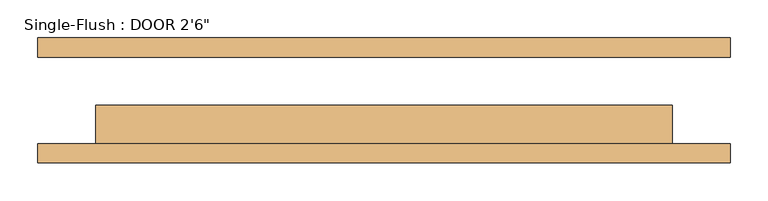
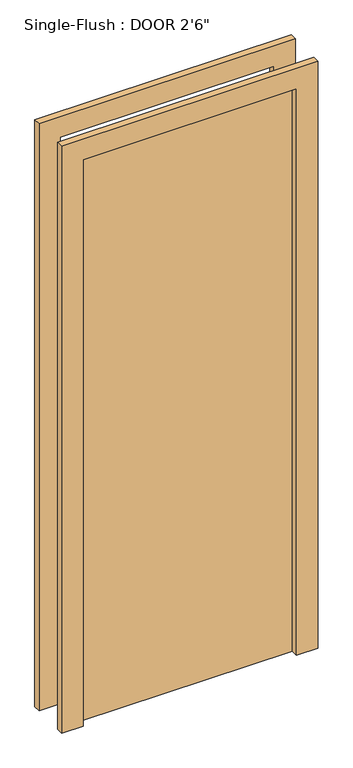
"""IFC4 building model written with IfcOpenShell, lengths in millimetres: door geometry."""

from ifc_helpers import new_model, si_unit, frame, origin, origin_with_axes, place, context, project, spatial, polyline, outline, extrude, source, transform, mapped, element, save


def door_78caadf7(model_context):
    return source(origin(), model_context, "Body", "SweptSolid", [
        extrude(outline(polyline([(2209.8, -457.2), (0.0, -457.2), (0.0, -381.0), (2133.6, -381.0), (2133.6, 381.0), (0.0, 381.0), (0.0, 457.2), (2209.8, 457.2), (2209.8, -457.2)])), frame((0.0, -82.55, 0.0), z_axis=(0.0, 1.0, 0.0), x_axis=(0.0, 0.0, 1.0)), (0.0, 0.0, 1.0), 25.4),
        extrude(outline(polyline([(2209.8, 457.2), (2209.8, -457.2), (0.0, -457.2), (0.0, -381.0), (2133.6, -381.0), (2133.6, 381.0), (0.0, 381.0), (0.0, 457.2), (2209.8, 457.2)])), frame((0.0, 57.15, 0.0), z_axis=(0.0, 1.0, 0.0), x_axis=(0.0, 0.0, 1.0)), (0.0, 0.0, 1.0), 25.4),
        extrude(outline(polyline([(381.0, -6.35), (381.0, -57.15), (-381.0, -57.15), (-381.0, -6.35), (381.0, -6.35)])), origin_with_axes(), (0.0, 0.0, 1.0), 2133.6),
    ])


if __name__ == "__main__":
    model = new_model("IFC4")
    model_context = context("Model", 3, world=origin())
    ifc_project = project(units=[si_unit("LENGTHUNIT", "METRE", prefix="MILLI")], contexts=[model_context])
    site = spatial("IfcSite", under=ifc_project)
    building = spatial("IfcBuilding", under=site)
    placement = place(None, origin())
    door_shape = door_78caadf7(model_context)
    element("IfcDoor", 1, ObjectType="Single-Flush : DOOR 2'6\"", at=placement, inside=building, context=model_context, shape_type="MappedRepresentation", body=[
        mapped(door_shape, transform((0.0, 0.0, 0.0), x_axis=(1.0, 0.0, 0.0), y_axis=(0.0, 1.0, 0.0), z_axis=(0.0, 0.0, 1.0))),
    ])
    save(model, "model.ifc")

# Revit data of these elements
# Type "Single-Flush : DOOR 2'6\""
#   Type Mark = "10"
#   Construction Type Id = "MDOOR"
#   Assembly Code = "C1020"
#   Analytic Construction = "Metal"
#   Thickness = 0' - 2"
#   Heat Transfer Coefficient (U) = 0.651978 BTU/(h·ft²·°F)
#   Height = 7' - 0"
#   Trim Projection Ext = 0' - 1"
#   Trim Projection Int = 0' - 1"
#   Trim Width = 0' - 3"
#   Width = 2' - 6"
#   Define Thermal Properties by = 1
#   Door Material = Door - Panel
#   Frame Material = Door - Frame
#   Visual Light Transmittance = 0
#   Solar Heat Gain Coefficient = 0
#   Function = (empty or 0)
#   Wall Closure = (empty or 0)
# Element 1 (IfcDoor, "Single-Flush : DOOR 2'6\"")
#   Materials on its faces: "Door - Frame", "Door - Panel"
# Materials
#   "Door - Panel": class "Wood", colour RGB 210 159 95, transparency 0, Cost = 0
#   "Door - Frame": colour RGB 118 70 51, transparency 0, Cost = 0
